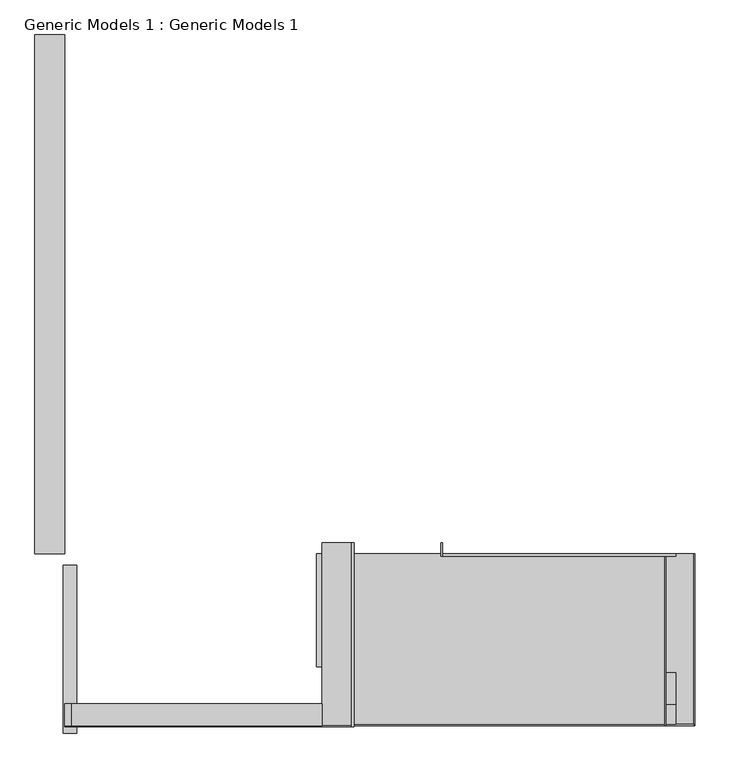
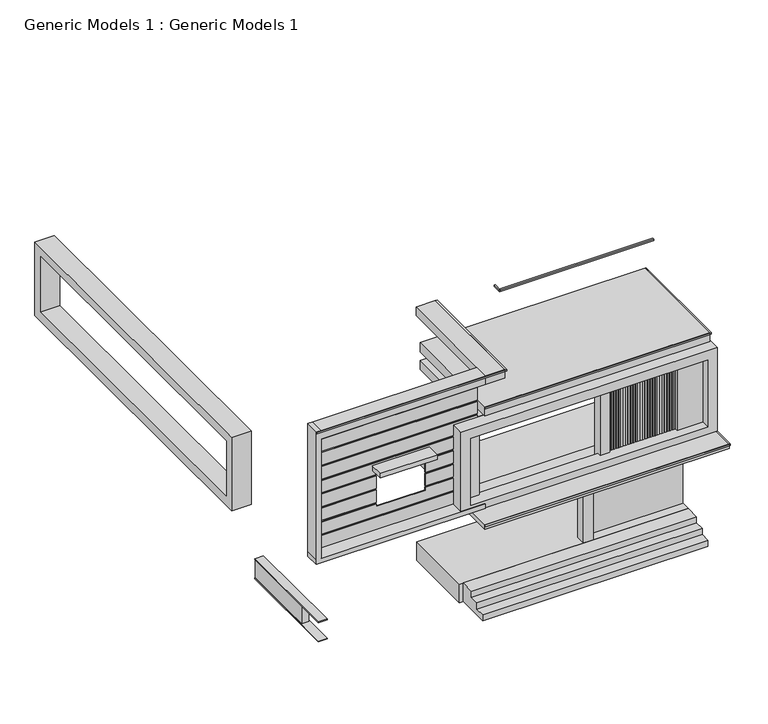
"""IFC4 building model written with IfcOpenShell, lengths in millimetres: proxy geometry, Generic Models 1 : Generic Models 1."""

from ifc_helpers import new_model, si_unit, frame, origin, origin_with_axes, place, context, project, spatial, polyline, outline, extrude, faceted_brep, source, transform, mapped, element, save


def generic_models_1_generic_models_1_72e2fdcd(model_context):
    return source(origin(), model_context, "Body", "SolidModel", [
        extrude(outline(polyline([(919.7837859, -6034.9648025), (919.7837859, -6060.3648025), (886.7566288, -6060.3648025), (886.7566288, -6034.9648025), (919.7837859, -6034.9648025)])), frame((0.0, 0.0, 4064.0), z_axis=(0.0, 0.0, 1.0), x_axis=(1.0, 0.0, 0.0)), (0.0, 0.0, 1.0), 2209.8),
        extrude(outline(polyline([(734.3566288, -6034.9648025), (785.1566288, -6034.9648025), (785.1566288, -6060.3648025), (734.3566288, -6060.3648025), (734.3566288, -6034.9648025)])), frame((0.0, 0.0, 4064.0), z_axis=(0.0, 0.0, 1.0), x_axis=(1.0, 0.0, 0.0)), (0.0, 0.0, 1.0), 2209.8),
        extrude(outline(polyline([(658.1566288, -6034.9648025), (708.9566288, -6034.9648025), (708.9566288, -6060.3648025), (658.1566288, -6060.3648025), (658.1566288, -6034.9648025)])), frame((0.0, 0.0, 4064.0), z_axis=(0.0, 0.0, 1.0), x_axis=(1.0, 0.0, 0.0)), (0.0, 0.0, 1.0), 2209.8),
        extrude(outline(polyline([(581.9566288, -6034.9648025), (632.7566288, -6034.9648025), (632.7566288, -6060.3648025), (581.9566288, -6060.3648025), (581.9566288, -6034.9648025)])), frame((0.0, 0.0, 4064.0), z_axis=(0.0, 0.0, 1.0), x_axis=(1.0, 0.0, 0.0)), (0.0, 0.0, 1.0), 2209.8),
        extrude(outline(polyline([(505.7566288, -6034.9648025), (556.5566288, -6034.9648025), (556.5566288, -6060.3648025), (505.7566288, -6060.3648025), (505.7566288, -6034.9648025)])), frame((0.0, 0.0, 4064.0), z_axis=(0.0, 0.0, 1.0), x_axis=(1.0, 0.0, 0.0)), (0.0, 0.0, 1.0), 2209.8),
        extrude(outline(polyline([(429.5566288, -6034.9648025), (480.3566288, -6034.9648025), (480.3566288, -6060.3648025), (429.5566288, -6060.3648025), (429.5566288, -6034.9648025)])), frame((0.0, 0.0, 4064.0), z_axis=(0.0, 0.0, 1.0), x_axis=(1.0, 0.0, 0.0)), (0.0, 0.0, 1.0), 2209.8),
        extrude(outline(polyline([(353.3566288, -6034.9648025), (404.1566288, -6034.9648025), (404.1566288, -6060.3648025), (353.3566288, -6060.3648025), (353.3566288, -6034.9648025)])), frame((0.0, 0.0, 4064.0), z_axis=(0.0, 0.0, 1.0), x_axis=(1.0, 0.0, 0.0)), (0.0, 0.0, 1.0), 2209.8),
        extrude(outline(polyline([(277.1566288, -6034.9648025), (327.9566288, -6034.9648025), (327.9566288, -6060.3648025), (277.1566288, -6060.3648025), (277.1566288, -6034.9648025)])), frame((0.0, 0.0, 4064.0), z_axis=(0.0, 0.0, 1.0), x_axis=(1.0, 0.0, 0.0)), (0.0, 0.0, 1.0), 2209.8),
        extrude(outline(polyline([(200.9566288, -6034.9648025), (251.7566288, -6034.9648025), (251.7566288, -6060.3648025), (200.9566288, -6060.3648025), (200.9566288, -6034.9648025)])), frame((0.0, 0.0, 4064.0), z_axis=(0.0, 0.0, 1.0), x_axis=(1.0, 0.0, 0.0)), (0.0, 0.0, 1.0), 2209.8),
        extrude(outline(polyline([(124.7566288, -6034.9648025), (175.5566288, -6034.9648025), (175.5566288, -6060.3648025), (124.7566288, -6060.3648025), (124.7566288, -6034.9648025)])), frame((0.0, 0.0, 4064.0), z_axis=(0.0, 0.0, 1.0), x_axis=(1.0, 0.0, 0.0)), (0.0, 0.0, 1.0), 2209.8),
        extrude(outline(polyline([(48.5566288, -6034.9648025), (99.3566288, -6034.9648025), (99.3566288, -6060.3648025), (48.5566288, -6060.3648025), (48.5566288, -6034.9648025)])), frame((0.0, 0.0, 4064.0), z_axis=(0.0, 0.0, 1.0), x_axis=(1.0, 0.0, 0.0)), (0.0, 0.0, 1.0), 2209.8),
        extrude(outline(polyline([(-27.6433712, -6034.9648025), (23.1566288, -6034.9648025), (23.1566288, -6060.3648025), (-27.6433712, -6060.3648025), (-27.6433712, -6034.9648025)])), frame((0.0, 0.0, 4064.0), z_axis=(0.0, 0.0, 1.0), x_axis=(1.0, 0.0, 0.0)), (0.0, 0.0, 1.0), 2209.8),
        extrude(outline(polyline([(-103.8433712, -6034.9648025), (-53.0433712, -6034.9648025), (-53.0433712, -6060.3648025), (-103.8433712, -6060.3648025), (-103.8433712, -6034.9648025)])), frame((0.0, 0.0, 4064.0), z_axis=(0.0, 0.0, 1.0), x_axis=(1.0, 0.0, 0.0)), (0.0, 0.0, 1.0), 2209.8),
        extrude(outline(polyline([(-180.0433712, -6034.9648025), (-129.2433712, -6034.9648025), (-129.2433712, -6060.3648025), (-180.0433712, -6060.3648025), (-180.0433712, -6034.9648025)])), frame((0.0, 0.0, 4064.0), z_axis=(0.0, 0.0, 1.0), x_axis=(1.0, 0.0, 0.0)), (0.0, 0.0, 1.0), 2209.8),
        extrude(outline(polyline([(-256.2433712, -6034.9648025), (-205.4433712, -6034.9648025), (-205.4433712, -6060.3648025), (-256.2433712, -6060.3648025), (-256.2433712, -6034.9648025)])), frame((0.0, 0.0, 4064.0), z_axis=(0.0, 0.0, 1.0), x_axis=(1.0, 0.0, 0.0)), (0.0, 0.0, 1.0), 2209.8),
        extrude(outline(polyline([(-332.4433712, -6034.9648025), (-281.6433712, -6034.9648025), (-281.6433712, -6060.3648025), (-332.4433712, -6060.3648025), (-332.4433712, -6034.9648025)])), frame((0.0, 0.0, 4064.0), z_axis=(0.0, 0.0, 1.0), x_axis=(1.0, 0.0, 0.0)), (0.0, 0.0, 1.0), 2209.8),
        extrude(outline(polyline([(-408.6433712, -6034.9648025), (-357.8433712, -6034.9648025), (-357.8433712, -6060.3648025), (-408.6433712, -6060.3648025), (-408.6433712, -6034.9648025)])), frame((0.0, 0.0, 4064.0), z_axis=(0.0, 0.0, 1.0), x_axis=(1.0, 0.0, 0.0)), (0.0, 0.0, 1.0), 2209.8),
        extrude(outline(polyline([(-484.8433712, -6034.9648025), (-434.0433712, -6034.9648025), (-434.0433712, -6060.3648025), (-484.8433712, -6060.3648025), (-484.8433712, -6034.9648025)])), frame((0.0, 0.0, 4064.0), z_axis=(0.0, 0.0, 1.0), x_axis=(1.0, 0.0, 0.0)), (0.0, 0.0, 1.0), 2209.8),
        extrude(outline(polyline([(-561.0433712, -6034.9648025), (-510.2433712, -6034.9648025), (-510.2433712, -6060.3648025), (-561.0433712, -6060.3648025), (-561.0433712, -6034.9648025)])), frame((0.0, 0.0, 4064.0), z_axis=(0.0, 0.0, 1.0), x_axis=(1.0, 0.0, 0.0)), (0.0, 0.0, 1.0), 2209.8),
        extrude(outline(polyline([(-637.2433712, -6034.9648025), (-586.4433712, -6034.9648025), (-586.4433712, -6060.3648025), (-637.2433712, -6060.3648025), (-637.2433712, -6034.9648025)])), frame((0.0, 0.0, 4064.0), z_axis=(0.0, 0.0, 1.0), x_axis=(1.0, 0.0, 0.0)), (0.0, 0.0, 1.0), 2209.8),
        extrude(outline(polyline([(-713.4433712, -6034.9648025), (-662.6433712, -6034.9648025), (-662.6433712, -6060.3648025), (-713.4433712, -6060.3648025), (-713.4433712, -6034.9648025)])), frame((0.0, 0.0, 4064.0), z_axis=(0.0, 0.0, 1.0), x_axis=(1.0, 0.0, 0.0)), (0.0, 0.0, 1.0), 2209.8),
        extrude(outline(polyline([(-789.6433712, -6034.9648025), (-738.8433712, -6034.9648025), (-738.8433712, -6060.3648025), (-789.6433712, -6060.3648025), (-789.6433712, -6034.9648025)])), frame((0.0, 0.0, 4064.0), z_axis=(0.0, 0.0, 1.0), x_axis=(1.0, 0.0, 0.0)), (0.0, 0.0, 1.0), 2209.8),
        extrude(outline(polyline([(-865.8433712, -6034.9648025), (-815.0433712, -6034.9648025), (-815.0433712, -6060.3648025), (-865.8433712, -6060.3648025), (-865.8433712, -6034.9648025)])), frame((0.0, 0.0, 4064.0), z_axis=(0.0, 0.0, 1.0), x_axis=(1.0, 0.0, 0.0)), (0.0, 0.0, 1.0), 2209.8),
        extrude(outline(polyline([(-942.0433712, -6034.9648025), (-891.2433712, -6034.9648025), (-891.2433712, -6060.3648025), (-942.0433712, -6060.3648025), (-942.0433712, -6034.9648025)])), frame((0.0, 0.0, 4064.0), z_axis=(0.0, 0.0, 1.0), x_axis=(1.0, 0.0, 0.0)), (0.0, 0.0, 1.0), 2209.8),
        extrude(outline(polyline([(-1018.2433712, -6034.9648025), (-967.4433712, -6034.9648025), (-967.4433712, -6060.3648025), (-1018.2433712, -6060.3648025), (-1018.2433712, -6034.9648025)])), frame((0.0, 0.0, 4064.0), z_axis=(0.0, 0.0, 1.0), x_axis=(1.0, 0.0, 0.0)), (0.0, 0.0, 1.0), 2209.8),
        extrude(outline(polyline([(-1094.4433712, -6034.9648025), (-1043.6433712, -6034.9648025), (-1043.6433712, -6060.3648025), (-1094.4433712, -6060.3648025), (-1094.4433712, -6034.9648025)])), frame((0.0, 0.0, 4064.0), z_axis=(0.0, 0.0, 1.0), x_axis=(1.0, 0.0, 0.0)), (0.0, 0.0, 1.0), 2209.8),
        extrude(outline(polyline([(-1170.6433712, -6034.9648025), (-1119.8433712, -6034.9648025), (-1119.8433712, -6060.3648025), (-1170.6433712, -6060.3648025), (-1170.6433712, -6034.9648025)])), frame((0.0, 0.0, 4064.0), z_axis=(0.0, 0.0, 1.0), x_axis=(1.0, 0.0, 0.0)), (0.0, 0.0, 1.0), 2209.8),
        extrude(outline(polyline([(810.5566288, -6034.9648025), (861.3566288, -6034.9648025), (861.3566288, -6060.3648025), (810.5566288, -6060.3648025), (810.5566288, -6034.9648025)])), frame((0.0, 0.0, 4064.0), z_axis=(0.0, 0.0, 1.0), x_axis=(1.0, 0.0, 0.0)), (0.0, 0.0, 1.0), 2209.8),
        faceted_brep([(-1476.7561572, -6126.9538441, 6308.1762568), (-1171.9561572, -6126.9538441, 6308.1762568), (-1171.9561572, -5822.1538441, 6308.1762568), (-1476.7561572, -5822.1538441, 6308.1762568), (-1476.7561572, -6126.9538441, 3810.0), (-1476.7561572, -5822.1538441, 3810.0), (-1171.9561572, -5822.1538441, 3810.0), (-1171.9561572, -6126.9538441, 3810.0), (-1171.9561572, -6060.3648025, 4064.0), (-1171.9561572, -6060.3648025, 6273.8), (-1171.9561572, -6034.9648025, 6273.8), (-1171.9561572, -6034.9648025, 4064.0), (-1196.0433712, -6060.3648025, 4064.0), (-1196.0433712, -6060.3648025, 6273.8), (-1196.0433712, -6034.9648025, 6273.8), (-1196.0433712, -6034.9648025, 4064.0)], [[[0, 1, 2, 3]], [[4, 5, 6, 7]], [[1, 0, 4, 7]], [[2, 1, 7, 6], [8, 9, 10, 11]], [[3, 2, 6, 5]], [[0, 3, 5, 4]], [[12, 13, 9, 8]], [[14, 15, 11, 10]], [[13, 14, 10, 9]], [[13, 12, 15, 14]], [[15, 12, 8, 11]]]),
        extrude(outline(polyline([(7769.9351975, 3657.6), (-2898.0648025, 3657.6), (-2898.0648025, 6096.0), (7769.9351975, 6096.0), (7769.9351975, 3657.6)]), holes=[polyline([(7465.1351975, 5791.2), (-2593.2648025, 5791.2), (-2593.2648025, 3962.4), (7465.1351975, 3962.4), (7465.1351975, 5791.2)])]), frame((-11153.7909398, 0.0, 0.0), z_axis=(1.0, 0.0, 0.0), x_axis=(0.0, 1.0, 0.0)), (0.0, 0.0, 1.0), 609.6),
        extrude(outline(polyline([(-2797.1909398, -2948.8648025), (-2797.1909398, -2669.4648025), (-2771.7909398, -2669.4648025), (-2771.7909398, -2948.8648025), (-2797.1909398, -2948.8648025)])), frame((0.0, 0.0, 8026.4), z_axis=(0.0, 0.0, 1.0), x_axis=(1.0, 0.0, 0.0)), (0.0, 0.0, 1.0), 50.8),
        extrude(outline(polyline([(1825.6090602, -2898.0648025), (1825.6090602, -6429.0796421), (1800.2090602, -6429.0796421), (1800.2090602, -2898.0648025), (1825.6090602, -2898.0648025)])), frame((0.0, 0.0, 7112.0), z_axis=(0.0, 0.0, 1.0), x_axis=(1.0, 0.0, 0.0)), (0.0, 0.0, 1.0), 50.8),
        extrude(outline(polyline([(2028.8090602, -2948.8648025), (-2771.7909398, -2948.8648025), (-2771.7909398, -2898.0648025), (2028.8090602, -2898.0648025), (2028.8090602, -2948.8648025)])), frame((0.0, 0.0, 8026.4), z_axis=(0.0, 0.0, 1.0), x_axis=(1.0, 0.0, 0.0)), (0.0, 0.0, 1.0), 50.8),
        extrude(outline(polyline([(1800.2090602, -6403.6796421), (-5248.2909398, -6403.6796421), (-5248.2909398, -2898.0648025), (1800.2090602, -2898.0648025), (1800.2090602, -6403.6796421)])), frame((0.0, 0.0, 6858.0), z_axis=(0.0, 0.0, 1.0), x_axis=(1.0, 0.0, 0.0)), (0.0, 0.0, 1.0), 304.8),
        extrude(outline(polyline([(-5248.2909398, -6101.2380415), (-5698.4993283, -6101.2380415), (-5698.4993283, -5999.6380415), (-5248.2909398, -5999.6380415), (-5248.2909398, -6101.2380415)])), frame((0.0, 0.0, 4064.0), z_axis=(0.0, 0.0, 1.0), x_axis=(1.0, 0.0, 0.0)), (0.0, 0.0, 1.0), 2209.8),
        extrude(outline(polyline([(6578.6, 2028.8090602), (6578.6, -6003.2993283), (3810.0, -6003.2993283), (3810.0, 2028.8090602), (6578.6, 2028.8090602)]), holes=[polyline([(6273.8, 1724.0090602), (4064.0, 1724.0090602), (4064.0, -5698.4993283), (6273.8, -5698.4993283), (6273.8, 1724.0090602)])]), frame((0.0, -6403.6796421, 0.0), z_axis=(0.0, 1.0, 0.0), x_axis=(0.0, 0.0, 1.0)), (0.0, 0.0, 1.0), 404.0416006),
        extrude(outline(polyline([(-5248.2909398, -5999.6380415), (-10391.7909398, -5999.6380415), (-10391.7909398, -5974.2380415), (-5248.2909398, -5974.2380415), (-5248.2909398, -5999.6380415)])), frame((0.0, 0.0, 7609.7801837), z_axis=(0.0, 0.0, 1.0), x_axis=(1.0, 0.0, 0.0)), (0.0, 0.0, 1.0), 315.0198163),
        extrude(outline(polyline([(3962.4, -10391.7909398), (3962.4, -5248.2909398), (4815.7801837, -5248.2909398), (4815.7801837, -6886.5909398), (4724.4, -6886.5909398), (4724.4, -8410.5909398), (4815.7801837, -8410.5909398), (4815.7801837, -10391.7909398), (4409.3801837, -10391.7909398), (4409.3801837, -6003.2993283), (4358.5801837, -6003.2993283), (4358.5801837, -10391.7909398), (3962.4, -10391.7909398)])), frame((0.0, -5999.6380415, 0.0), z_axis=(0.0, 1.0, 0.0), x_axis=(0.0, 0.0, 1.0)), (0.0, 0.0, 1.0), 25.4),
        extrude(outline(polyline([(5969.0, -8410.5909398), (5969.0, -6886.5909398), (5780.9801837, -6886.5909398), (5780.9801837, -5248.2909398), (6187.3801837, -5248.2909398), (6187.3801837, -10391.7909398), (5780.9801837, -10391.7909398), (5780.9801837, -8410.5909398), (5969.0, -8410.5909398)])), frame((0.0, -5999.6380415, 0.0), z_axis=(0.0, 1.0, 0.0), x_axis=(0.0, 0.0, 1.0)), (0.0, 0.0, 1.0), 25.4),
        extrude(outline(polyline([(-5248.2909398, -5999.6380415), (-10391.7909398, -5999.6380415), (-10391.7909398, -5974.2380415), (-5248.2909398, -5974.2380415), (-5248.2909398, -5999.6380415)])), frame((0.0, 0.0, 7152.5801837), z_axis=(0.0, 0.0, 1.0), x_axis=(1.0, 0.0, 0.0)), (0.0, 0.0, 1.0), 406.4),
        extrude(outline(polyline([(-5248.2909398, -5999.6380415), (-10391.7909398, -5999.6380415), (-10391.7909398, -5974.2380415), (-5248.2909398, -5974.2380415), (-5248.2909398, -5999.6380415)])), frame((0.0, 0.0, 6695.3801837), z_axis=(0.0, 0.0, 1.0), x_axis=(1.0, 0.0, 0.0)), (0.0, 0.0, 1.0), 406.4),
        extrude(outline(polyline([(-5248.2909398, -5999.6380415), (-10391.7909398, -5999.6380415), (-10391.7909398, -5974.2380415), (-5248.2909398, -5974.2380415), (-5248.2909398, -5999.6380415)])), frame((0.0, 0.0, 6238.1801837), z_axis=(0.0, 0.0, 1.0), x_axis=(1.0, 0.0, 0.0)), (0.0, 0.0, 1.0), 406.4),
        extrude(outline(polyline([(-8410.5909398, -5999.6380415), (-10391.7909398, -5999.6380415), (-10391.7909398, -5974.2380415), (-8410.5909398, -5974.2380415), (-8410.5909398, -5999.6380415)])), frame((0.0, 0.0, 5323.7801837), z_axis=(0.0, 0.0, 1.0), x_axis=(1.0, 0.0, 0.0)), (0.0, 0.0, 1.0), 406.4),
        extrude(outline(polyline([(-8410.5909398, -5999.6380415), (-10391.7909398, -5999.6380415), (-10391.7909398, -5974.2380415), (-8410.5909398, -5974.2380415), (-8410.5909398, -5999.6380415)])), frame((0.0, 0.0, 4866.5801837), z_axis=(0.0, 0.0, 1.0), x_axis=(1.0, 0.0, 0.0)), (0.0, 0.0, 1.0), 406.4),
        extrude(outline(polyline([(-5248.2909398, -5999.6380415), (-6886.5909398, -5999.6380415), (-6886.5909398, -5974.2380415), (-5248.2909398, -5974.2380415), (-5248.2909398, -5999.6380415)])), frame((0.0, 0.0, 5323.7801837), z_axis=(0.0, 0.0, 1.0), x_axis=(1.0, 0.0, 0.0)), (0.0, 0.0, 1.0), 406.4),
        extrude(outline(polyline([(-5248.2909398, -5999.6380415), (-6886.5909398, -5999.6380415), (-6886.5909398, -5974.2380415), (-5248.2909398, -5974.2380415), (-5248.2909398, -5999.6380415)])), frame((0.0, 0.0, 4866.5801837), z_axis=(0.0, 0.0, 1.0), x_axis=(1.0, 0.0, 0.0)), (0.0, 0.0, 1.0), 406.4),
        faceted_brep([(-10544.1909398, -6431.4380415, 3810.0), (-5248.2909398, -6431.4380415, 3810.0), (-5248.2909398, -6431.4380415, 3962.4), (-10391.7909398, -6431.4380415, 3962.4), (-10391.7909398, -6431.4380415, 7924.8), (-5248.2909398, -6431.4380415, 7924.8), (-5248.2909398, -6431.4380415, 8204.2), (-10391.7909398, -6431.4380415, 8204.2), (-10544.1909398, -6431.4380415, 8204.2), (-10544.1909398, -6431.4380415, 3962.4), (-10544.1909398, -5974.2380415, 3810.0), (-10544.1909398, -5974.2380415, 3962.4), (-10544.1909398, -5974.2380415, 8204.2), (-10391.7909398, -5974.2380415, 8204.2), (-5248.2909398, -5974.2380415, 8204.2), (-5248.2909398, -5974.2380415, 7924.8), (-10391.7909398, -5974.2380415, 7924.8), (-10391.7909398, -5974.2380415, 7609.7801837), (-10391.7909398, -5974.2380415, 7558.9801837), (-10391.7909398, -5974.2380415, 7152.5801837), (-10391.7909398, -5974.2380415, 7101.7801837), (-10391.7909398, -5974.2380415, 6695.3801837), (-10391.7909398, -5974.2380415, 6644.5801837), (-10391.7909398, -5974.2380415, 6238.1801837), (-10391.7909398, -5974.2380415, 6187.3801837), (-10391.7909398, -5974.2380415, 5780.9801837), (-10391.7909398, -5974.2380415, 5730.1801837), (-10391.7909398, -5974.2380415, 5323.7801837), (-10391.7909398, -5974.2380415, 5272.9801837), (-10391.7909398, -5974.2380415, 4866.5801837), (-10391.7909398, -5974.2380415, 4815.7801837), (-10391.7909398, -5974.2380415, 4409.3801837), (-10391.7909398, -5974.2380415, 4358.5801837), (-10391.7909398, -5974.2380415, 3962.4), (-5248.2909398, -5974.2380415, 3962.4), (-5248.2909398, -5974.2380415, 3810.0)], [[[0, 1, 2, 3, 4, 5, 6, 7, 8, 9]], [[10, 11, 12, 13, 14, 15, 16, 17, 18, 19, 20, 21, 22, 23, 24, 25, 26, 27, 28, 29, 30, 31, 32, 33, 34, 35]], [[1, 0, 10, 35]], [[2, 1, 35, 34]], [[3, 2, 34, 33]], [[4, 3, 33, 32, 31, 30, 29, 28, 27, 26, 25, 24, 23, 22, 21, 20, 19, 18, 17, 16]], [[5, 4, 16, 15]], [[6, 5, 15, 14]], [[7, 6, 14, 13]], [[8, 7, 13, 12]], [[9, 8, 12, 11]], [[0, 9, 11, 10]]]),
        extrude(outline(polyline([(1800.2090602, -6429.0796421), (-5248.2909398, -6429.0796421), (-5248.2909398, -6403.6796421), (1800.2090602, -6403.6796421), (1800.2090602, -6429.0796421)])), frame((0.0, 0.0, 7112.0), z_axis=(0.0, 0.0, 1.0), x_axis=(1.0, 0.0, 0.0)), (0.0, 0.0, 1.0), 50.8),
        extrude(outline(polyline([(-4587.8909398, -2669.4648025), (-4587.8909398, -6456.8380415), (-4638.6909398, -6456.8380415), (-4638.6909398, -2669.4648025), (-4587.8909398, -2669.4648025)])), frame((0.0, 0.0, 8153.4), z_axis=(0.0, 0.0, 1.0), x_axis=(1.0, 0.0, 0.0)), (0.0, 0.0, 1.0), 50.8),
        extrude(outline(polyline([(-4638.6909398, -6456.8380415), (-10544.1909398, -6456.8380415), (-10544.1909398, -6431.4380415), (-4638.6909398, -6431.4380415), (-4638.6909398, -6456.8380415)])), frame((0.0, 0.0, 8153.4), z_axis=(0.0, 0.0, 1.0), x_axis=(1.0, 0.0, 0.0)), (0.0, 0.0, 1.0), 50.8),
        extrude(outline(polyline([(-4638.6909398, -2669.4648025), (-4638.6909398, -6431.4380415), (-5248.2909398, -6431.4380415), (-5248.2909398, -2669.4648025), (-4638.6909398, -2669.4648025)])), frame((0.0, 0.0, 7924.8), z_axis=(0.0, 0.0, 1.0), x_axis=(1.0, 0.0, 0.0)), (0.0, 0.0, 1.0), 279.4),
        extrude(outline(polyline([(-5248.2909398, -2898.0648025), (1800.2090602, -2898.0648025), (1800.2090602, -5999.6380415), (-5248.2909398, -5999.6380415), (-5248.2909398, -2898.0648025)])), frame((0.0, 0.0, 6273.8), z_axis=(0.0, 0.0, 1.0), x_axis=(1.0, 0.0, 0.0)), (0.0, 0.0, 1.0), 304.8),
        extrude(outline(polyline([(2028.8090602, -5999.6380415), (-5248.2909398, -5999.6380415), (-5248.2909398, -5336.4648025), (2028.8090602, -5336.4648025), (2028.8090602, -5999.6380415)])), frame((0.0, 0.0, 3657.6), z_axis=(0.0, 0.0, 1.0), x_axis=(1.0, 0.0, 0.0)), (0.0, 0.0, 1.0), 152.4),
        extrude(outline(polyline([(919.7837859, -6151.8887846), (919.7837859, -6060.3648025), (1724.0090602, -6060.3648025), (1724.0090602, -6151.8887846), (919.7837859, -6151.8887846)])), frame((0.0, 0.0, 4064.0), z_axis=(0.0, 0.0, 1.0), x_axis=(1.0, 0.0, 0.0)), (0.0, 0.0, 1.0), 2209.8),
        extrude(outline(polyline([(-6759.5909398, -6431.4380415), (-8537.5909398, -6431.4380415), (-8537.5909398, -5974.2380415), (-6759.5909398, -5974.2380415), (-6759.5909398, -6431.4380415)])), frame((0.0, 0.0, 5969.0), z_axis=(0.0, 0.0, 1.0), x_axis=(1.0, 0.0, 0.0)), (0.0, 0.0, 1.0), 152.4),
        extrude(outline(polyline([(-5222.1648025, 609.9098343), (-5222.1648025, 0.3098343), (-6279.0380415, 0.3098343), (-6279.0380415, 203.5098343), (-5974.2380415, 203.5098343), (-5974.2380415, 406.7098343), (-5669.4380415, 406.7098343), (-5669.4380415, 609.9098343), (-5222.1648025, 609.9098343)])), frame((-5248.2909398, 0.0, 0.0), z_axis=(1.0, 0.0, 0.0), x_axis=(0.0, 1.0, 0.0)), (0.0, 0.0, 1.0), 7048.5),
        extrude(outline(polyline([(-10544.1909398, -5641.2648025), (-10544.1909398, -3127.1231213), (-10315.5909398, -3127.1231213), (-10315.5909398, -5641.2648025), (-10544.1909398, -5641.2648025)])), frame((0.0, 0.0, 1371.6), z_axis=(0.0, 0.0, 1.0), x_axis=(1.0, 0.0, 0.0)), (0.0, 0.0, 1.0), 609.6),
        extrude(outline(polyline([(-10290.1909398, -6581.0648025), (-10569.5909398, -6581.0648025), (-10569.5909398, -3130.2170173), (-10290.1909398, -3130.2170173), (-10290.1909398, -6581.0648025)])), frame((0.0, 0.0, 1981.2), z_axis=(0.0, 0.0, 1.0), x_axis=(1.0, 0.0, 0.0)), (0.0, 0.0, 1.0), 25.4),
        extrude(outline(polyline([(-10569.5909398, -6581.0648025), (-10569.5909398, -3130.2170173), (-10290.1909398, -3130.2170173), (-10290.1909398, -6581.0648025), (-10569.5909398, -6581.0648025)])), frame((0.0, 0.0, 1346.2), z_axis=(0.0, 0.0, 1.0), x_axis=(1.0, 0.0, 0.0)), (0.0, 0.0, 1.0), 25.4),
        extrude(outline(polyline([(2395.4304038, -6429.0796421), (-5248.2909398, -6429.0796421), (-5248.2909398, -6403.6796421), (2395.4304038, -6403.6796421), (2395.4304038, -6429.0796421)])), frame((0.0, 0.0, 3209.3762568), z_axis=(0.0, 0.0, 1.0), x_axis=(1.0, 0.0, 0.0)), (0.0, 0.0, 1.0), 50.8),
        extrude(outline(polyline([(2420.8304038, -2898.0648025), (2420.8304038, -6429.0796421), (2395.4304038, -6429.0796421), (2395.4304038, -2898.0648025), (2420.8304038, -2898.0648025)])), frame((0.0, 0.0, 3209.3762568), z_axis=(0.0, 0.0, 1.0), x_axis=(1.0, 0.0, 0.0)), (0.0, 0.0, 1.0), 50.8),
        extrude(outline(polyline([(1800.2090602, -4907.7538441), (1800.2090602, -4933.1538441), (-1171.9561572, -4933.1538441), (-1171.9561572, -4907.7538441), (1800.2090602, -4907.7538441)])), frame((0.0, 0.0, 609.6), z_axis=(0.0, 0.0, 1.0), x_axis=(1.0, 0.0, 0.0)), (0.0, 0.0, 1.0), 2498.1762568),
        extrude(outline(polyline([(-1476.7561572, -5212.5538441), (-1476.7561572, -4907.7538441), (-1171.9561572, -4907.7538441), (-1171.9561572, -5212.5538441), (-1476.7561572, -5212.5538441)])), frame((0.0, 0.0, 609.6), z_axis=(0.0, 0.0, 1.0), x_axis=(1.0, 0.0, 0.0)), (0.0, 0.0, 1.0), 2498.1762568),
        extrude(outline(polyline([(2395.4304038, -6403.6796421), (-5248.2909398, -6403.6796421), (-5248.2909398, -2898.0648025), (2395.4304038, -2898.0648025), (2395.4304038, -6403.6796421)])), frame((0.0, 0.0, 3107.7762568), z_axis=(0.0, 0.0, 1.0), x_axis=(1.0, 0.0, 0.0)), (0.0, 0.0, 1.0), 152.4),
        extrude(outline(polyline([(1800.2090602, -5222.1648025), (-5362.5909398, -5222.1648025), (-5362.5909398, -2898.0648025), (1800.2090602, -2898.0648025), (1800.2090602, -5222.1648025)])), origin_with_axes(), (0.0, 0.0, 1.0), 609.6),
    ])


if __name__ == "__main__":
    model = new_model("IFC4")
    model_context = context("Model", 3, world=origin())
    ifc_project = project(units=[si_unit("LENGTHUNIT", "METRE", prefix="MILLI")], contexts=[model_context])
    site = spatial("IfcSite", under=ifc_project)
    building = spatial("IfcBuilding", under=site)
    placement = place(None, origin())
    generic_models_1_generic_models_1_shape = generic_models_1_generic_models_1_72e2fdcd(model_context)
    element("IfcBuildingElementProxy", 1, Name="Generic Models 1 : Generic Models 1", ObjectType="Generic Models 1 : Generic Models 1", at=placement, inside=building, context=model_context, shape_type="MappedRepresentation", body=[
        mapped(generic_models_1_generic_models_1_shape, transform((0.0, 0.0, 0.0), x_axis=(1.0, 0.0, 0.0), y_axis=(0.0, 1.0, 0.0), z_axis=(0.0, 0.0, 1.0))),
    ])
    save(model, "model.ifc")

# Revit data of these elements
# Element 1 (IfcBuildingElementProxy, "Generic Models 1 : Generic Models 1")
#   Materials on its faces: "wood", "Laminate, Ivory, Matte", "window wall", "balcony extrusion", "Gypsum Wall Board", "tile"
# Materials
#   "wood": class "Generic", colour RGB 120 120 120, transparency 0, Cost = 0
#   "Laminate, Ivory, Matte": class "Plastic", colour RGB 247 247 239, transparency 0, Description = "Plastic Laminate - Ivory, Matte", Cost = 0
#   "window wall": class "Generic", colour RGB 120 120 120, transparency 0, Cost = 0
#   "balcony extrusion": class "Generic", colour RGB 120 120 120, transparency 0, Cost = 0
#   "Gypsum Wall Board": class "Generic", colour RGB 127 127 127, transparency 0, Description = "Gypsum Wall Board", Cost = 0
#   "tile": class "Generic", colour RGB 120 120 120, transparency 0, Cost = 0
